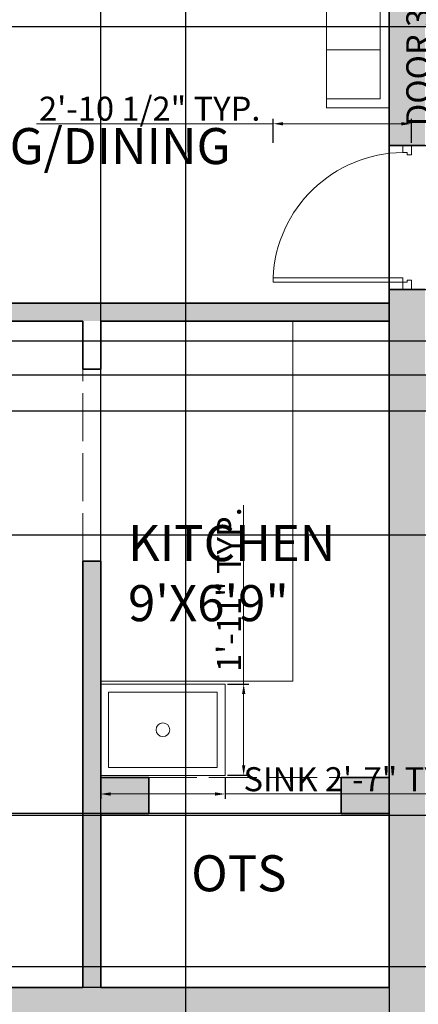
# Model space of a CAD drawing. Units: inches. Extents: x 2696 to 3240, y 1564 to 2310.
# Tile 24 of 76: x 2864 to 2964, y 1736 to 1982. Entities that reach past the tile are written whole.
import ezdxf

# ---------------------------------------------------------------- set-up
doc = ezdxf.new("R2010")
doc.units = ezdxf.units.IN
doc.linetypes.add('ACAD_ISO02W100', pattern=[15, 12, -3])
for name, color, linetype, lineweight in [('A-ANNO-DIMS', 3, 'Continuous', 18), ('A-AREA-IDEN', 7, 'Continuous', 18), ('A-DOOR', 4, 'Continuous', 18), ('A-FLOR-CASE', 8, 'Continuous', 18), ('A-FLOR-FIXT', 8, 'Continuous', 18), ('A-FURN', 251, 'Continuous', 13), ('A-WALL', 7, 'Continuous', 35), ('A-WALL-OVHD', 7, 'ACAD_ISO02W100', 18), ('A-WALL-PATT', 9, 'Continuous', 13)]:
    doc.layers.add(name, color=color, linetype=linetype, lineweight=lineweight)
doc.styles.add('TIMES NEW', font='times.ttf')
doc.styles.add('YQ_DIM', font='SUPEROS.SHX', dxfattribs={"width": 0.8, "bigfont": 'HZDX.SHX'})
doc.dimstyles.new('Siddhuu', dxfattribs={"dimtxt": 6, "dimasz": 2.5, "dimexe": 1.25, "dimexo": 0.625, "dimtad": 1, "dimdec": 1, "dimlunit": 4, "dimtxsty": 'TIMES NEW', "dimcen": 2.5, "dimclrd": 256, "dimclre": 1, "dimclrt": 7, "dimadec": 0, "dimazin": 0, "dimtfac": 1, "dimtdec": 1, "dimtmove": 0, "dimatfit": 3, "dimfxl": 1, "dimtolj": 1, "dimlwd": -1, "dimarcsym": 0})

# ---------------------------------------------------------------- blocks, each defined once
blk = doc.blocks.new('DR_D01')
for p, q in [((-0.45, 0.93), (-0.42, 0.93)), ((-0.45, 0.03), (-0.45, 0.93)), ((-0.42, 0.03), (-0.42, 0.93)), ((-0.5, 0.03), (-0.42, 0.03)), ((-0.5, 0.03), (-0.5, -0.03)), ((-0.45, 0.03), (-0.45, 0)), ((-0.45, 0), (-0.435, 0)), ((-0.435, 0), (-0.435, -0.03)), ((0.435, 0), (0.435, -0.03)), ((0.45, 0), (0.435, 0)), ((0.45, 0.03), (0.45, 0)), ((0.5, 0.03), (0.45, 0.03)), ((0.5, -0.03), (0.5, 0.03)), ((-0.435, -0.03), (-0.5, -0.03)), ((0.435, -0.03), (0.5, -0.03))]:
    blk.add_line(p, q)
blk.add_arc((-0.4602, 0.0206), 0.9103, 0.59152, 87.46644)
blk = doc.blocks.new('SOFA-SECTIONAL')
for p, q in [((0, 43.61), (0, 59.26)), ((0, 59.26), (58.14, 59.26)), ((58.14, 59.26), (58.14, 0)), ((2.24, 43.61), (2.24, 57.02)), ((2.24, 57.02), (55.9, 57.02)), ((13.42, 57.02), (13.42, 43.61)), ((27.95, 57.02), (27.95, 43.61)), ((42.49, 57.02), (42.49, 0)), ((55.9, 57.02), (55.9, 2.24)), ((0, 43.61), (55.9, 43.61)), ((42.49, 29.07), (55.9, 29.07)), ((42.49, 14.54), (55.9, 14.54)), ((55.9, 2.24), (42.49, 2.24)), ((58.14, 0), (42.49, 0))]:
    blk.add_line(p, q)
blk = doc.blocks.new('SINK-KITCHEN')
for points in [[(0, 22.8), (31.04, 22.8), (31.04, 0), (0, 0)], [(1.97, 20.82), (29.07, 20.82), (29.07, 1.97), (1.97, 1.97)]]:
    blk.add_lwpolyline(points, close=True)
blk.add_circle((15.52, 11.4), 1.71)
blk = doc.blocks.new('*D30')
at = {"layer": 'A-ANNO-DIMS', "transparency": 16777216}
for p, q in [((2967.69, 1950.58), (2967.69, 2019.05)), ((2967.69, 1917.08), (2967.69, 1948.08))]:
    blk.add_line(p, q, dxfattribs=at)
at = {"layer": 'A-ANNO-DIMS', "color": 1, "lineweight": -2, "transparency": 16777216}
for p, q in [((2962.91, 1950.58), (2968.94, 1950.58)), ((2962.91, 1914.58), (2968.94, 1914.58))]:
    blk.add_line(p, q, dxfattribs=at)
at = {"layer": 'A-ANNO-DIMS', "transparency": 16777216}
for points in [[(2967.27, 1948.08), (2968.11, 1948.08), (2967.69, 1950.58)], [(2967.27, 1917.08), (2968.11, 1917.08), (2967.69, 1914.58)]]:
    blk.add_solid(points, dxfattribs=at)
at = {"layer": 'Defpoints', "color": 0, "transparency": 16777216}
for p in [(2962.29, 1950.58), (2967.69, 1950.58), (2962.29, 1914.58)]:
    blk.add_point(p, dxfattribs=at)
at = {"layer": 'A-ANNO-DIMS', "color": 7, "transparency": 16777216, "insert": (2964, 1986.06), "char_height": 6, "attachment_point": 5, "rotation": 90, "style": 'TIMES NEW'}
blk.add_mtext('\\A1;DOOR 3\'-0" TYP.', dxfattribs=at)
blk = doc.blocks.new('*D31')
at = {"layer": 'A-ANNO-DIMS', "transparency": 16777216}
for p, q in [((2927.73, 1955.98), (2868.64, 1955.98)), ((2959.79, 1955.98), (2930.23, 1955.98))]:
    blk.add_line(p, q, dxfattribs=at)
at = {"layer": 'A-ANNO-DIMS', "color": 1, "lineweight": -2, "transparency": 16777216}
for p, q in [((2927.73, 1951.2), (2927.73, 1957.23)), ((2962.29, 1951.2), (2962.29, 1957.23))]:
    blk.add_line(p, q, dxfattribs=at)
at = {"layer": 'A-ANNO-DIMS', "transparency": 16777216}
for points in [[(2930.23, 1956.39), (2930.23, 1955.56), (2927.73, 1955.98)], [(2959.79, 1956.39), (2959.79, 1955.56), (2962.29, 1955.98)]]:
    blk.add_solid(points, dxfattribs=at)
at = {"layer": 'Defpoints', "color": 0, "transparency": 16777216}
for p in [(2927.73, 1955.98), (2927.73, 1950.58), (2962.29, 1950.58)]:
    blk.add_point(p, dxfattribs=at)
at = {"layer": 'A-ANNO-DIMS', "color": 7, "transparency": 16777216, "insert": (2896.94, 1959.74), "char_height": 6, "attachment_point": 5, "style": 'TIMES NEW'}
blk.add_mtext('\\A1;2\'-10 1/2" TYP.', dxfattribs=at)
blk = doc.blocks.new('*D42')
at = {"layer": 'A-ANNO-DIMS', "color": 1, "lineweight": -2, "transparency": 16777216}
for p, q in [((2884.71, 1792.59), (2884.71, 1787.31)), ((2915.75, 1792.59), (2915.75, 1787.31))]:
    blk.add_line(p, q, dxfattribs=at)
at = {"layer": 'A-ANNO-DIMS', "transparency": 16777216}
for p, q in [((2887.21, 1788.56), (2913.25, 1788.56)), ((2915.75, 1788.56), (2979.39, 1788.56))]:
    blk.add_line(p, q, dxfattribs=at)
for points in [[(2887.21, 1788.98), (2887.21, 1788.14), (2884.71, 1788.56)], [(2913.25, 1788.98), (2913.25, 1788.14), (2915.75, 1788.56)]]:
    blk.add_solid(points, dxfattribs=at)
at = {"layer": 'Defpoints', "color": 0, "transparency": 16777216}
for p in [(2884.71, 1793.22), (2915.75, 1793.22), (2915.75, 1788.56)]:
    blk.add_point(p, dxfattribs=at)
at = {"layer": 'A-ANNO-DIMS', "color": 7, "transparency": 16777216, "insert": (2948.82, 1792.25), "char_height": 6, "attachment_point": 5, "style": 'TIMES NEW'}
blk.add_mtext('\\A1;SINK 2\'-7" TYP.', dxfattribs=at)
blk = doc.blocks.new('*D43')
at = {"layer": 'A-ANNO-DIMS', "transparency": 16777216}
for p, q in [((2920.4, 1816.01), (2920.4, 1860.71)), ((2920.4, 1795.72), (2920.4, 1813.51))]:
    blk.add_line(p, q, dxfattribs=at)
at = {"layer": 'A-ANNO-DIMS', "color": 1, "lineweight": -2, "transparency": 16777216}
for p, q in [((2916.37, 1816.01), (2921.65, 1816.01)), ((2916.37, 1793.22), (2921.65, 1793.22))]:
    blk.add_line(p, q, dxfattribs=at)
at = {"layer": 'A-ANNO-DIMS', "transparency": 16777216}
for points in [[(2919.99, 1813.51), (2920.82, 1813.51), (2920.4, 1816.01)], [(2919.99, 1795.72), (2920.82, 1795.72), (2920.4, 1793.22)]]:
    blk.add_solid(points, dxfattribs=at)
at = {"layer": 'Defpoints', "color": 0, "transparency": 16777216}
for p in [(2915.75, 1816.01), (2920.4, 1816.01), (2915.75, 1793.22)]:
    blk.add_point(p, dxfattribs=at)
at = {"layer": 'A-ANNO-DIMS', "color": 7, "transparency": 16777216, "insert": (2916.72, 1839.61), "char_height": 6, "attachment_point": 5, "rotation": 90, "style": 'TIMES NEW'}
blk.add_mtext('\\A1;1\'-11" TYP.', dxfattribs=at)
blk = doc.blocks.new('*D55')
at = {"layer": 'A-ANNO-DIMS', "color": 1, "lineweight": -2, "transparency": 16777216}
for p, q in [((3189.99, 1980.2), (2709.36, 1980.2)), ((3189.99, 1893.2), (2709.36, 1893.2))]:
    blk.add_line(p, q, dxfattribs=at)
at = {"layer": 'A-ANNO-DIMS', "transparency": 16777216}
blk.add_line((2710.61, 1895.7), (2710.61, 1977.7), dxfattribs=at)
for points in [[(2710.19, 1977.7), (2711.03, 1977.7), (2710.61, 1980.2)], [(2710.19, 1895.7), (2711.03, 1895.7), (2710.61, 1893.2)]]:
    blk.add_solid(points, dxfattribs=at)
at = {"layer": 'Defpoints', "color": 0, "transparency": 16777216}
for p in [(2710.61, 1980.2), (3190.61, 1980.2), (3190.61, 1893.2)]:
    blk.add_point(p, dxfattribs=at)
at = {"layer": 'A-ANNO-DIMS', "color": 7, "transparency": 16777216, "insert": (2706.93, 1936.7), "char_height": 6, "attachment_point": 5, "rotation": 90, "style": 'TIMES NEW'}
blk.add_mtext('\\A1;7\'-3"', dxfattribs=at)
blk = doc.blocks.new('*D57')
at = {"layer": 'A-ANNO-DIMS', "color": 1, "lineweight": -2, "transparency": 16777216}
for p, q in [((2754.61, 2018.58), (2754.61, 1568.95)), ((2956.71, 2018.58), (2956.71, 1568.95))]:
    blk.add_line(p, q, dxfattribs=at)
at = {"layer": 'A-ANNO-DIMS', "transparency": 16777216}
blk.add_line((2757.11, 1570.2), (2954.21, 1570.2), dxfattribs=at)
for points in [[(2757.11, 1570.62), (2757.11, 1569.78), (2754.61, 1570.2)], [(2954.21, 1570.62), (2954.21, 1569.78), (2956.71, 1570.2)]]:
    blk.add_solid(points, dxfattribs=at)
at = {"layer": 'Defpoints', "color": 0, "transparency": 16777216}
for p in [(2754.61, 2019.2), (2956.71, 2019.2), (2956.71, 1570.2)]:
    blk.add_point(p, dxfattribs=at)
at = {"layer": 'A-ANNO-DIMS', "color": 7, "transparency": 16777216, "insert": (2855.66, 1573.88), "char_height": 6, "attachment_point": 5, "style": 'TIMES NEW'}
blk.add_mtext('\\A1;16\'-10"', dxfattribs=at)
blk = doc.blocks.new('*D59')
at = {"layer": 'A-ANNO-DIMS', "color": 1, "lineweight": -2, "transparency": 16777216}
for p, q in [((2884.71, 1740.83), (2884.71, 2298.45)), ((2956.71, 1740.83), (2956.71, 2298.45))]:
    blk.add_line(p, q, dxfattribs=at)
at = {"layer": 'A-ANNO-DIMS', "transparency": 16777216}
blk.add_line((2887.21, 2297.2), (2954.21, 2297.2), dxfattribs=at)
for points in [[(2887.21, 2297.62), (2887.21, 2296.78), (2884.71, 2297.2)], [(2954.21, 2297.62), (2954.21, 2296.78), (2956.71, 2297.2)]]:
    blk.add_solid(points, dxfattribs=at)
at = {"layer": 'Defpoints', "color": 0, "transparency": 16777216}
for p in [(2956.71, 2297.2), (2884.71, 1740.2), (2956.71, 1740.2)]:
    blk.add_point(p, dxfattribs=at)
at = {"layer": 'A-ANNO-DIMS', "color": 7, "transparency": 16777216, "insert": (2920.71, 2300.88), "char_height": 6, "attachment_point": 5, "style": 'TIMES NEW'}
blk.add_mtext('\\A1;6\'-0"', dxfattribs=at)
blk = doc.blocks.new('*D60')
at = {"layer": 'A-ANNO-DIMS', "color": 1, "lineweight": -2, "transparency": 16777216}
for p, q in [((2956.08, 1783.7), (2709.36, 1783.7)), ((2956.08, 1740.2), (2709.36, 1740.2))]:
    blk.add_line(p, q, dxfattribs=at)
at = {"layer": 'A-ANNO-DIMS', "transparency": 16777216}
blk.add_line((2710.61, 1742.7), (2710.61, 1781.2), dxfattribs=at)
for points in [[(2710.19, 1781.2), (2711.03, 1781.2), (2710.61, 1783.7)], [(2710.19, 1742.7), (2711.03, 1742.7), (2710.61, 1740.2)]]:
    blk.add_solid(points, dxfattribs=at)
at = {"layer": 'Defpoints', "color": 0, "transparency": 16777216}
for p in [(2710.61, 1783.7), (2956.71, 1783.7), (2956.71, 1740.2)]:
    blk.add_point(p, dxfattribs=at)
at = {"layer": 'A-ANNO-DIMS', "color": 7, "transparency": 16777216, "insert": (2706.85, 1761.95), "char_height": 6, "attachment_point": 5, "rotation": 90, "style": 'TIMES NEW'}
blk.add_mtext('\\A1;3\'-7 1/2"', dxfattribs=at)
blk = doc.blocks.new('*D69')
at = {"layer": 'A-ANNO-DIMS', "color": 1, "lineweight": -2, "transparency": 16777216}
for p, q in [((2841.89, 2261.58), (2841.89, 1568.95)), ((2905.91, 2261.58), (2905.91, 1568.95))]:
    blk.add_line(p, q, dxfattribs=at)
at = {"layer": 'A-ANNO-DIMS', "transparency": 16777216}
blk.add_line((2844.39, 1570.2), (2903.41, 1570.2), dxfattribs=at)
for points in [[(2844.39, 1570.62), (2844.39, 1569.78), (2841.89, 1570.2)], [(2903.41, 1570.62), (2903.41, 1569.78), (2905.91, 1570.2)]]:
    blk.add_solid(points, dxfattribs=at)
at = {"layer": 'Defpoints', "color": 0, "transparency": 16777216}
for p in [(2841.89, 2262.2), (2905.91, 2262.2), (2905.91, 1570.2)]:
    blk.add_point(p, dxfattribs=at)
at = {"layer": 'A-ANNO-DIMS', "color": 7, "transparency": 16777216, "insert": (2873.9, 1573.88), "char_height": 6, "attachment_point": 5, "style": 'TIMES NEW'}
blk.add_mtext('\\A1;5\'-4"', dxfattribs=at)
blk = doc.blocks.new('*D78')
at = {"layer": 'A-ANNO-DIMS', "transparency": 16777216}
for p, q in [((2710.61, 1901.7), (2710.61, 1935.1)), ((2710.61, 1895.7), (2710.61, 1899.2))]:
    blk.add_line(p, q, dxfattribs=at)
at = {"layer": 'A-ANNO-DIMS', "color": 1, "lineweight": -2, "transparency": 16777216}
for p, q in [((3189.99, 1901.7), (2709.36, 1901.7)), ((3189.99, 1893.2), (2709.36, 1893.2))]:
    blk.add_line(p, q, dxfattribs=at)
at = {"layer": 'A-ANNO-DIMS', "transparency": 16777216}
for points in [[(2710.19, 1899.2), (2711.03, 1899.2), (2710.61, 1901.7)], [(2710.19, 1895.7), (2711.03, 1895.7), (2710.61, 1893.2)]]:
    blk.add_solid(points, dxfattribs=at)
at = {"layer": 'Defpoints', "color": 0, "transparency": 16777216}
for p in [(2710.61, 1901.7), (3190.61, 1901.7), (3190.61, 1893.2)]:
    blk.add_point(p, dxfattribs=at)
at = {"layer": 'A-ANNO-DIMS', "color": 7, "transparency": 16777216, "insert": (2706.85, 1919.65), "char_height": 6, "attachment_point": 5, "rotation": 90, "style": 'TIMES NEW'}
blk.add_mtext('\\A1;0\'-8 1/2"', dxfattribs=at)
blk = doc.blocks.new('*D79')
at = {"layer": 'A-ANNO-DIMS', "color": 1, "lineweight": -2, "transparency": 16777216}
for p, q in [((3189.99, 1884.2), (2709.36, 1884.2)), ((3189.99, 1853.2), (2709.36, 1853.2))]:
    blk.add_line(p, q, dxfattribs=at)
at = {"layer": 'A-ANNO-DIMS', "transparency": 16777216}
blk.add_line((2710.61, 1881.7), (2710.61, 1855.7), dxfattribs=at)
for points in [[(2710.19, 1881.7), (2711.03, 1881.7), (2710.61, 1884.2)], [(2710.19, 1855.7), (2711.03, 1855.7), (2710.61, 1853.2)]]:
    blk.add_solid(points, dxfattribs=at)
at = {"layer": 'Defpoints', "color": 0, "transparency": 16777216}
for p in [(3190.61, 1884.2), (2710.61, 1853.2), (3190.61, 1853.2)]:
    blk.add_point(p, dxfattribs=at)
at = {"layer": 'A-ANNO-DIMS', "color": 7, "transparency": 16777216, "insert": (2706.93, 1868.7), "char_height": 6, "attachment_point": 5, "rotation": 90, "style": 'TIMES NEW'}
blk.add_mtext('\\A1;2\'-7"', dxfattribs=at)
blk = doc.blocks.new('*D80')
at = {"layer": 'A-ANNO-DIMS', "color": 1, "lineweight": -2, "transparency": 16777216}
for p, q in [((3198.99, 1783.2), (2709.36, 1783.2)), ((3198.99, 1745.35), (2709.36, 1745.35))]:
    blk.add_line(p, q, dxfattribs=at)
at = {"layer": 'A-ANNO-DIMS', "transparency": 16777216}
blk.add_line((2710.61, 1780.7), (2710.61, 1747.85), dxfattribs=at)
for points in [[(2710.19, 1780.7), (2711.03, 1780.7), (2710.61, 1783.2)], [(2710.19, 1747.85), (2711.03, 1747.85), (2710.61, 1745.35)]]:
    blk.add_solid(points, dxfattribs=at)
at = {"layer": 'Defpoints', "color": 0, "transparency": 16777216}
for p in [(3199.61, 1783.2), (2710.61, 1745.35), (3199.61, 1745.35)]:
    blk.add_point(p, dxfattribs=at)
at = {"layer": 'A-ANNO-DIMS', "color": 7, "transparency": 16777216, "insert": (2706.93, 1764.28), "char_height": 6, "attachment_point": 5, "rotation": 90, "style": 'TIMES NEW'}
blk.add_mtext('\\A1;3\'-2"', dxfattribs=at)

msp = doc.modelspace()

# ---------------------------------------------------------------- hatches: boundary and pattern name
at = {"layer": 'A-WALL-PATT', "transparency": 33554556}
h = msp.add_hatch(color=256, dxfattribs=at)
h.dxf.hatch_style = 1
h.paths.add_polyline_path([(2879.11, 2253.2), (2905.91, 2253.2), (2905.91, 2262.2), (2841.89, 2262.2), (2841.89, 2253.2), (2870.11, 2253.2), (2870.11, 2176.6), (2965.71, 2176.6), (2965.71, 2206.7), (2973.58, 2206.7), (2973.58, 2215.7), (2965.71, 2215.7), (2965.71, 2262.2), (2929.91, 2262.2), (2929.91, 2253.2), (2956.71, 2253.2), (2956.71, 2185.6), (2879.11, 2185.6)])
h.paths.add_polyline_path([(2782.83, 2262.2), (2745.61, 2262.2), (2745.61, 2228.73), (2754.61, 2228.73), (2754.61, 2253.2), (2782.83, 2253.2)])
h.paths.add_polyline_path([(2754.61, 2136.2), (2965.71, 2136.2), (2965.71, 2145.2), (2879.11, 2145.2), (2879.11, 2147.07), (2877.34, 2147.07), (2870.11, 2147.07), (2870.11, 2145.2), (2754.61, 2145.2), (2754.61, 2169.67), (2745.61, 2169.67), (2745.61, 2000.2), (2754.61, 2000.2), (2754.61, 2019.2), (2849.08, 2019.2), (2849.08, 2023.7), (2841.21, 2023.7), (2841.21, 2051.83), (2836.71, 2051.83), (2836.71, 2023.7), (2754.61, 2023.7), (2754.61, 2091.2), (2836.71, 2091.2), (2836.71, 2087.83), (2841.21, 2087.83), (2841.21, 2095.7), (2754.61, 2095.7)])
h.paths.add_polyline_path([(2965.71, 2136.2), (2956.71, 2136.2), (2956.71, 2023.7), (2885.08, 2023.7), (2885.08, 2019.2), (2956.71, 2019.2), (2956.71, 1950.58), (2965.71, 1950.58), (2965.71, 1980.2), (2973.58, 1980.2), (2973.58, 1989.2), (2965.71, 1989.2)])
h.paths.add_polyline_path([(2754.61, 1906.7), (2880.21, 1906.7), (2884.71, 1906.7), (2956.71, 1906.7), (2956.71, 1792.7), (2944.71, 1792.7), (2944.71, 1783.7), (2956.71, 1783.7), (2956.71, 1740.2), (2884.71, 1740.2), (2884.71, 1783.7), (2896.71, 1783.7), (2896.71, 1792.7), (2884.71, 1792.7), (2884.71, 1846.7), (2880.21, 1846.7), (2880.21, 1740.2), (2754.61, 1740.2), (2754.61, 1777.2), (2745.61, 1777.2), (2745.61, 1692.7), (2754.61, 1692.7), (2754.61, 1731.2), (2956.71, 1731.2), (2956.71, 1723.33), (2965.71, 1723.33), (2965.71, 1884.2), (2973.58, 1884.2), (2973.58, 1893.2), (2965.71, 1893.2), (2965.71, 1914.58), (2956.71, 1914.58), (2956.71, 1911.2), (2754.61, 1911.2), (2754.61, 1930.2), (2745.61, 1930.2), (2745.61, 1817.2), (2754.61, 1817.2), (2754.61, 1854.2), (2826.61, 1854.2), (2826.61, 1868.83), (2822.11, 1868.83), (2822.11, 1858.7), (2754.61, 1858.7)])
h.paths.add_polyline_path([(2965.71, 1656.2), (3008.24, 1656.2), (3008.24, 1665.2), (2965.71, 1665.2), (2965.71, 1693.33), (2956.71, 1693.33), (2956.71, 1686.2), (2934.58, 1686.2), (2934.58, 1681.7), (2956.71, 1681.7), (2956.71, 1614.2), (2896.71, 1614.2), (2896.71, 1681.7), (2904.58, 1681.7), (2904.58, 1686.2), (2892.21, 1686.2), (2892.21, 1614.2), (2858.41, 1614.2), (2858.41, 1605.2), (2965.71, 1605.2)])
h.paths.add_polyline_path([(2788.41, 1614.2), (2754.61, 1614.2), (2754.61, 1652.7), (2745.61, 1652.7), (2745.61, 1605.2), (2788.41, 1605.2)])
h.paths.add_polyline_path([(3199.61, 1633.05), (3190.61, 1633.05), (3190.61, 1614.2), (3082.61, 1614.2), (3082.61, 1665.2), (3070.24, 1665.2), (3070.24, 1656.2), (3078.11, 1656.2), (3078.11, 1605.2), (3199.61, 1605.2)])
h.paths.add_polyline_path([(3199.61, 1702.05), (3190.61, 1702.05), (3190.61, 1699.7), (3106.61, 1699.7), (3106.61, 1747.7), (3190.61, 1747.7), (3190.61, 1752.2), (3082.61, 1752.2), (3082.61, 1760.08), (3078.11, 1760.08), (3078.11, 1747.7), (3102.11, 1747.7), (3102.11, 1699.7), (3078.11, 1699.7), (3078.11, 1695.2), (3190.61, 1695.2), (3190.61, 1676.35), (3199.61, 1676.35)])
h.paths.add_polyline_path([(3199.61, 1783.2), (3190.61, 1783.2), (3190.61, 1745.35), (3199.61, 1745.35)])
h.paths.add_polyline_path([(3082.61, 1884.2), (3190.61, 1884.2), (3190.61, 1853.2), (3199.61, 1853.2), (3199.61, 1901.7), (3190.61, 1901.7), (3190.61, 1893.2), (3005.58, 1893.2), (3005.58, 1891.28), (3005.58, 1884.2), (3078.11, 1884.2), (3078.11, 1792.08), (3082.61, 1792.08)])
h.paths.add_polyline_path([(3199.61, 1994.7), (3190.61, 1994.7), (3190.61, 1989.2), (3073.71, 1989.2), (3073.71, 2034.2), (3069.21, 2034.2), (3069.21, 1989.2), (3005.58, 1989.2), (3005.58, 1980.2), (3190.61, 1980.2), (3190.61, 1971.7), (3199.61, 1971.7)])
h.paths.add_polyline_path([(3199.61, 2155.2), (3190.61, 2155.2), (3190.61, 2064.7), (3199.61, 2064.7)])
h.paths.add_polyline_path([(3190.61, 2074.7), (3106.61, 2074.7), (3106.61, 2122.7), (3190.61, 2122.7), (3190.61, 2127.2), (3082.71, 2127.2), (3082.71, 2135.08), (3073.71, 2135.08), (3073.71, 2122.7), (3102.11, 2122.7), (3102.11, 2074.7), (3069.21, 2074.7), (3069.21, 2070.2), (3190.61, 2070.2)])
h.paths.add_polyline_path([(3082.71, 2253.2), (3190.61, 2253.2), (3190.61, 2225.2), (3199.61, 2225.2), (3199.61, 2262.2), (3073.71, 2262.2), (3073.71, 2215.7), (3035.58, 2215.7), (3035.58, 2206.7), (3073.71, 2206.7), (3073.71, 2171.08), (3082.71, 2171.08)])

# ---------------------------------------------------------------- linework, layer by layer
at = {"layer": 'A-FLOR-CASE'}
for p in [(2932.71, 1906.7), (2884.71, 1816.7)]:
    msp.add_line(p, (2932.71, 1816.7), dxfattribs=at)
at = {"layer": 'A-WALL'}
for p, q in [((2956.71, 2019.2), (2956.71, 1950.58)), ((2965.71, 1950.58), (2956.71, 1950.58)), ((2956.71, 1914.58), (2956.71, 1911.2)), ((2965.71, 1914.58), (2956.71, 1914.58)), ((2754.61, 1911.2), (2956.71, 1911.2)), ((2754.61, 1906.7), (2880.21, 1906.7)), ((2880.21, 1906.7), (2880.21, 1894.7)), ((2884.71, 1906.7), (2884.71, 1894.7)), ((2884.71, 1906.7), (2956.71, 1906.7)), ((2956.71, 1906.7), (2956.71, 1792.7)), ((2880.21, 1894.7), (2884.71, 1894.7)), ((2880.21, 1846.7), (2884.71, 1846.7)), ((2880.21, 1846.7), (2880.21, 1740.2)), ((2884.71, 1846.7), (2884.71, 1792.7)), ((2884.71, 1792.7), (2896.71, 1792.7)), ((2896.71, 1783.7), (2896.71, 1792.7)), ((2944.71, 1783.7), (2944.71, 1792.7)), ((2944.71, 1792.7), (2956.71, 1792.7)), ((2884.71, 1783.7), (2896.71, 1783.7)), ((2884.71, 1783.7), (2884.71, 1740.2)), ((2944.71, 1783.7), (2956.71, 1783.7)), ((2956.71, 1783.7), (2956.71, 1740.2)), ((2754.61, 1740.2), (2880.21, 1740.2)), ((2884.71, 1740.2), (2956.71, 1740.2))]:
    msp.add_line(p, q, dxfattribs=at)
at = {"layer": 'A-WALL-OVHD'}
for p, q in [((2880.21, 1846.7), (2880.21, 1894.7)), ((2884.71, 1894.7), (2884.71, 1846.7)), ((2896.71, 1792.7), (2944.71, 1792.7)), ((2896.71, 1783.7), (2944.71, 1783.7))]:
    msp.add_line(p, q, dxfattribs=at)

# ---------------------------------------------------------------- block references
at = {"layer": 'A-DOOR', "xscale": 36, "yscale": 36, "zscale": 36, "rotation": 90}
msp.add_blockref('DR_D01', (2961.21, 1932.58), dxfattribs=at)
at = {"layer": 'A-FLOR-FIXT'}
msp.add_blockref('SINK-KITCHEN', (2884.71, 1793.21), dxfattribs=at)
at = {"layer": 'A-FURN'}
msp.add_blockref('SOFA-SECTIONAL', (2898.57, 1959.94), dxfattribs=at)

# ---------------------------------------------------------------- texts
at = {"layer": 'A-AREA-IDEN', "char_height": 9, "attachment_point": 1, "style": 'YQ_DIM'}
for s, width, insert in [('LIVING/DINING', 92.6128, (2832.18, 1954.9)), ('KITCHEN\\P9\'X6\'9"', 48.0032, (2891.53, 1855.73)), ('OTS', 48.0032, (2907.31, 1773.25))]:
    msp.add_mtext_dynamic_manual_height_columns(s, width=width, gutter_width=12.5, heights=[0], dxfattribs=dict(at, insert=insert))

# ---------------------------------------------------------------- dimensions: what is measured, and where the dimension line sits
at = {"layer": 'A-ANNO-DIMS'}
for base, p1, p2, picture, middle in [((2956.71, 2297.2), (2884.71, 1740.2), (2956.71, 1740.2), '*D59', (2920.71, 2300.88)), ((2905.91, 1570.2), (2841.89, 2262.2), (2905.91, 2262.2), '*D69', (2873.9, 1573.88)), ((2956.71, 1570.2), (2754.61, 2019.2), (2956.71, 2019.2), '*D57', (2855.66, 1573.88))]:
    dim = msp.add_linear_dim(base=base, p1=p1, p2=p2, dimstyle='Siddhuu', override={"dimdec": 1, "dimlfac": 1, "dimrnd": 0, "dimzin": 1, "dimdsep": 46, "dimlunit": 4, "dimfrac": 2}, dxfattribs=at)
    dim.commit()
    dim.dimension.update_dxf_attribs({"geometry": picture, "text_midpoint": middle})
for base, p1, p2, angle, text, picture, middle in [((2967.69, 1950.58), (2962.29, 1914.58), (2962.29, 1950.58), 90, 'DOOR <> TYP.', '*D30', (2964, 1986.06)), ((2927.73, 1955.98), (2962.29, 1950.58), (2927.73, 1950.58), 180, '<> TYP.', '*D31', (2896.94, 1959.74)), ((2920.4, 1816.01), (2915.75, 1793.21), (2915.75, 1816.01), 90, '<> TYP.', '*D43', (2916.72, 1839.61))]:
    dim = msp.add_linear_dim(base=base, p1=p1, p2=p2, angle=angle, text=text, dimstyle='Siddhuu', override={"dimdec": 1, "dimlfac": 1, "dimrnd": 0, "dimzin": 1, "dimdsep": 46, "dimlunit": 4, "dimfrac": 2}, dxfattribs=at)
    dim.commit()
    dim.dimension.update_dxf_attribs({"geometry": picture, "text_midpoint": middle})
for base, p1, p2, picture, middle in [((2710.61, 1980.2), (3190.61, 1893.2), (3190.61, 1980.2), '*D55', (2706.93, 1936.7)), ((2710.61, 1901.7), (3190.61, 1893.2), (3190.61, 1901.7), '*D78', (2706.85, 1919.65)), ((2710.61, 1853.2), (3190.61, 1884.2), (3190.61, 1853.2), '*D79', (2706.93, 1868.7)), ((2710.61, 1783.7), (2956.71, 1740.2), (2956.71, 1783.7), '*D60', (2706.85, 1761.95)), ((2710.6114, 1745.3546), (3199.6114, 1783.2011), (3199.6114, 1745.3546), '*D80', (2706.9345, 1764.2779))]:
    dim = msp.add_linear_dim(base=base, p1=p1, p2=p2, angle=90, dimstyle='Siddhuu', override={"dimdec": 1, "dimlfac": 1, "dimrnd": 0, "dimzin": 1, "dimdsep": 46, "dimlunit": 4, "dimfrac": 2}, dxfattribs=at)
    dim.commit()
    dim.dimension.update_dxf_attribs({"geometry": picture, "text_midpoint": middle})
dim = msp.add_linear_dim(base=(2915.75, 1788.56), p1=(2884.71, 1793.21), p2=(2915.75, 1793.21), text='SINK <> TYP.', dimstyle='Siddhuu', override={"dimdec": 1, "dimlfac": 1, "dimrnd": 0, "dimzin": 1, "dimdsep": 46, "dimlunit": 4, "dimfrac": 2}, dxfattribs=at)
dim.commit()
dim.dimension.update_dxf_attribs({"geometry": '*D42', "text_midpoint": (2948.82, 1792.25)})

doc.saveas('drawing.dxf')
